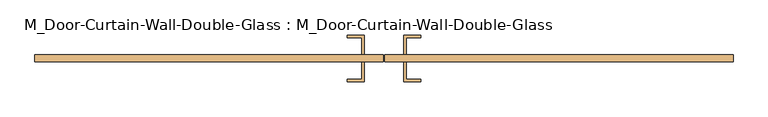
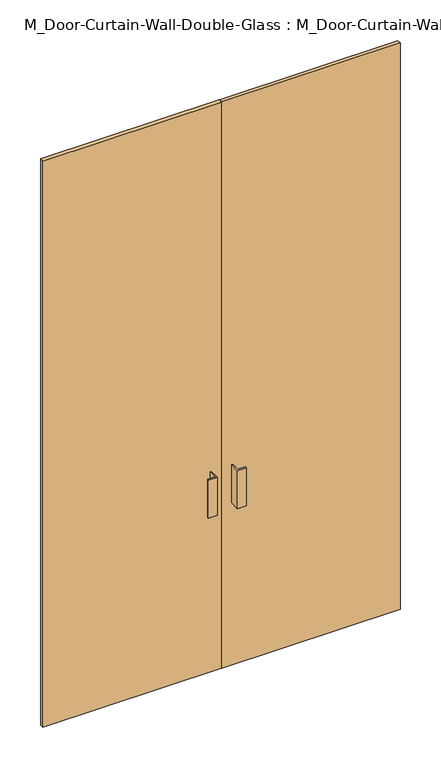
"""IFC4 building model written with IfcOpenShell, lengths in millimetres: door geometry, M_Door-Curtain-Wall-Double-Glass : M_Door-Curtain-Wall-Double-Glass."""

from ifc_helpers import new_model, si_unit, frame, origin, origin_with_axes, place, context, project, spatial, polyline, outline, extrude, source, transform, mapped, element, save


def m_door_curtain_wall_double_glass_m_door_curtain_wall_double_f99ce068(model_context):
    return source(origin(), model_context, "Body", "SweptSolid", [
        extrude(outline(polyline([(901.25, 31.75), (1.6106001, 31.75), (1.6106001, 50.8), (901.25, 50.8), (901.25, 31.75)])), origin_with_axes(), (0.0, 0.0, 1.0), 3020.0),
        extrude(outline(polyline([(-1.5643999, 31.75), (-901.25, 31.75), (-901.25, 50.8), (-1.5643999, 50.8), (-1.5643999, 31.75)])), origin_with_axes(), (0.0, 0.0, 1.0), 3020.0),
        extrude(outline(polyline([(-50.7768999, 101.6), (-50.7768999, 50.8), (-57.1268999, 50.8), (-57.1268999, 95.25), (-95.2268999, 95.25), (-95.2268999, 101.6), (-50.7768999, 101.6)])), frame((0.0, 0.0, 863.6), z_axis=(0.0, 0.0, 1.0), x_axis=(1.0, 0.0, 0.0)), (0.0, 0.0, 1.0), 203.2),
        extrude(outline(polyline([(50.8231001, 101.6), (95.2731001, 101.6), (95.2731001, 95.25), (57.1731001, 95.25), (57.1731001, 50.8), (50.8231001, 50.8), (50.8231001, 101.6)])), frame((0.0, 0.0, 863.6), z_axis=(0.0, 0.0, 1.0), x_axis=(1.0, 0.0, 0.0)), (0.0, 0.0, 1.0), 203.2),
        extrude(outline(polyline([(-50.7768999, -19.05), (-95.2268999, -19.05), (-95.2268999, -12.7), (-57.1268999, -12.7), (-57.1268999, 31.75), (-50.7768999, 31.75), (-50.7768999, -19.05)])), frame((0.0, 0.0, 863.6), z_axis=(0.0, 0.0, 1.0), x_axis=(1.0, 0.0, 0.0)), (0.0, 0.0, 1.0), 203.2),
        extrude(outline(polyline([(50.8231001, -19.05), (50.8231001, 31.75), (57.1731001, 31.75), (57.1731001, -12.7), (95.2731001, -12.7), (95.2731001, -19.05), (50.8231001, -19.05)])), frame((0.0, 0.0, 863.6), z_axis=(0.0, 0.0, 1.0), x_axis=(1.0, 0.0, 0.0)), (0.0, 0.0, 1.0), 203.2),
    ])


if __name__ == "__main__":
    model = new_model("IFC4")
    model_context = context("Model", 3, world=origin())
    ifc_project = project(units=[si_unit("LENGTHUNIT", "METRE", prefix="MILLI")], contexts=[model_context])
    site = spatial("IfcSite", under=ifc_project)
    building = spatial("IfcBuilding", under=site)
    placement = place(None, origin())
    m_door_curtain_wall_double_glass_m_door_curtain_wall_double_shape = m_door_curtain_wall_double_glass_m_door_curtain_wall_double_f99ce068(model_context)
    element("IfcDoor", 1, ObjectType="M_Door-Curtain-Wall-Double-Glass : M_Door-Curtain-Wall-Double-Glass", at=placement, inside=building, context=model_context, shape_type="MappedRepresentation", body=[
        mapped(m_door_curtain_wall_double_glass_m_door_curtain_wall_double_shape, transform((0.0, 0.0, 0.0), x_axis=(1.0, 0.0, 0.0), y_axis=(0.0, 1.0, 0.0), z_axis=(0.0, 0.0, 1.0))),
    ])
    save(model, "model.ifc")

# Revit data of these elements
# Type "M_Door-Curtain-Wall-Double-Glass : M_Door-Curtain-Wall-Double-Glass"
#   Type Mark = "53"
#   Assembly Code = "B2030100"
#   Analytic Construction = "<None>"
#   Width [instance default] = 1800 mm
#   Thermal Resistance (R) = 1.7611 (m²·K)/W
#   Swing Angle [instance default] = 90.00°
#   Panel Width [instance default] = 900 mm
#   Offset = 50.8 mm
#   Heat Transfer Coefficient (U) = 0.567826 W/(m²·K)
#   Define Thermal Properties by = 1
#   Function = 1
#   Door Handle Material = Aluminum
#   Glazing = Glass
#   Visual Light Transmittance = 0
#   Solar Heat Gain Coefficient = 0
#   Construction Type Id = ""
# Element 1 (IfcDoor, "M_Door-Curtain-Wall-Double-Glass : M_Door-Curtain-Wall-Double-Glass")
#   Width = 1802.5 mm
#   Panel Width = 901.25 mm
#   Materials on its faces: "Aluminum", "Glass"
# Materials
#   "Aluminum": class "Metal", colour RGB 244 245 246, transparency 0, Description = "Aluminum 6061", Cost = 0
#   "Glass": class "Glass", colour RGB 245 245 243, transparency 1, Description = "Soda Lime Glass", Cost = 0
